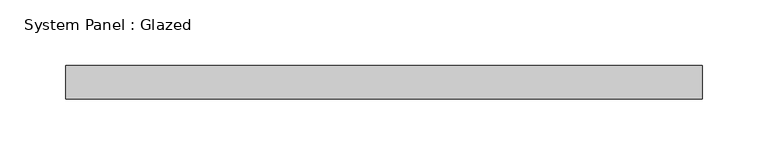
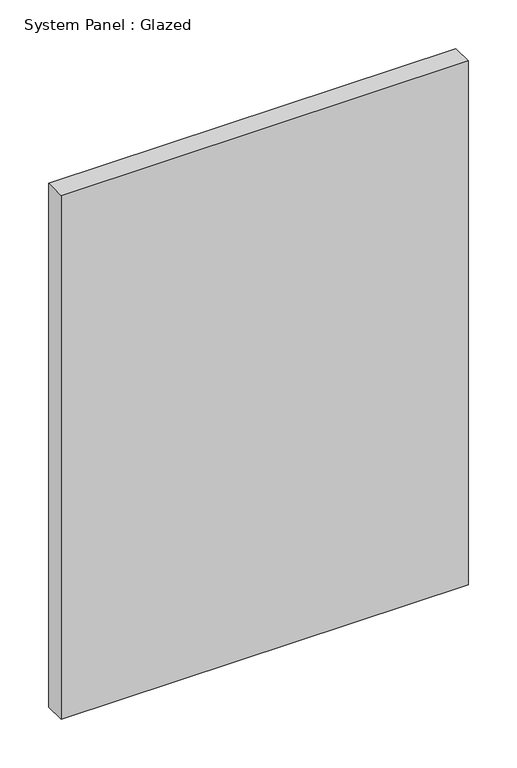
"""IFC4 building model written with IfcOpenShell, lengths in millimetres: plate geometry, System Panel : Glazed."""

from ifc_helpers import new_model, si_unit, origin, origin_with_axes, place, context, project, spatial, polyline, outline, extrude, source, transform, mapped, element, save


def system_panel_glazed_76104635(model_context):
    return source(origin(), model_context, "Body", "SweptSolid", [
        extrude(outline(polyline([(241.3, 19.05), (-241.3, 19.05), (-241.3, 44.45), (241.3, 44.45), (241.3, 19.05)])), origin_with_axes(), (0.0, 0.0, 1.0), 656.3085391),
    ])


if __name__ == "__main__":
    model = new_model("IFC4")
    model_context = context("Model", 3, world=origin())
    ifc_project = project(units=[si_unit("LENGTHUNIT", "METRE", prefix="MILLI")], contexts=[model_context])
    site = spatial("IfcSite", under=ifc_project)
    building = spatial("IfcBuilding", under=site)
    placement = place(None, origin())
    system_panel_glazed_shape = system_panel_glazed_76104635(model_context)
    element("IfcPlate", 1, ObjectType="System Panel : Glazed", at=placement, inside=building, context=model_context, shape_type="MappedRepresentation", body=[
        mapped(system_panel_glazed_shape, transform((0.0, 0.0, 0.0), x_axis=(1.0, 0.0, 0.0), y_axis=(0.0, 1.0, 0.0), z_axis=(0.0, 0.0, 1.0))),
    ])
    save(model, "model.ifc")

# Revit data of these elements
# Type "System Panel : Glazed"
#   Construction Type Id = "GSP4R"
#   Analytic Construction = "1/8 in Pilkington single glazing"
#   Visual Light Transmittance = 0.9
#   Solar Heat Gain Coefficient = 0.86
#   Heat Transfer Coefficient (U) = 1.18115 BTU/(h·ft²·°F)
#   Define Thermal Properties by = 1
# Element 1 (IfcPlate, "System Panel : Glazed")
#   Materials on its faces: "Glass"
# Materials
#   "Glass": class "Glass", colour RGB 0 128 192, transparency 0.75, Description = "Soda Lime Glass", Cost = 0
